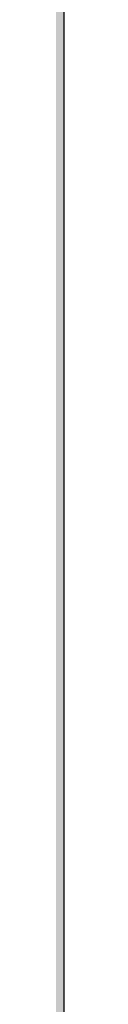
# Model space of a CAD drawing. Units: inches. Extents: x 2091 to 2899, y 967 to 2217.
# Tile 72 of 256: x 2212.144 to 2212.144, y 1102.499 to 1105.165. Entities that reach past the tile are written whole.
import ezdxf

# ---------------------------------------------------------------- set-up
doc = ezdxf.new("R2010")
doc.units = ezdxf.units.IN
doc.layers.add('A-ANNO-DIMS', color=2, linetype='Continuous', lineweight=18)
doc.layers.add('A-WALL-PATT', color=141, linetype='Continuous', lineweight=13, true_color=0xadddf7)
doc.styles.get("Standard").update_dxf_attribs({"font": 'arial.ttf'})
doc.dimstyles.new('ISO-25', dxfattribs={"dimtxt": 4, "dimasz": 4, "dimexe": 1.25, "dimexo": 0.625, "dimtad": 1, "dimdec": 0, "dimlunit": 3, "dimtxsty": 'Standard', "dimcen": 2.5, "dimadec": 0, "dimazin": 0, "dimtfac": 1, "dimtdec": 0, "dimtmove": 0, "dimatfit": 3, "dimfxl": 1, "dimarcsym": 0})

# ---------------------------------------------------------------- blocks, each defined once
blk = doc.blocks.new('*D71')
at = {"layer": 'A-ANNO-DIMS', "color": 0, "lineweight": -2, "transparency": 16777216}
for p, q in [((2212.1436, 1351.2941), (2212.1436, 969.4643)), ((2452.1436, 1351.2941), (2452.1436, 969.4643)), ((2216.1436, 970.7143), (2448.1436, 970.7143))]:
    blk.add_line(p, q, dxfattribs=at)
at = {"layer": 'A-ANNO-DIMS', "color": 0, "transparency": 16777216}
for points in [[(2216.1436, 971.381), (2216.1436, 970.0476), (2212.1436, 970.7143)], [(2448.1436, 971.381), (2448.1436, 970.0476), (2452.1436, 970.7143)]]:
    blk.add_solid(points, dxfattribs=at)
at = {"layer": 'Defpoints', "color": 0, "transparency": 16777216}
for p in [(2212.1436, 1351.9191), (2452.1436, 1351.9191), (2452.1436, 970.7143)]:
    blk.add_point(p, dxfattribs=at)
at = {"layer": 'A-ANNO-DIMS', "color": 0, "transparency": 16777216, "insert": (2332.1436, 973.3816), "char_height": 4, "attachment_point": 5}
blk.add_mtext('20\'-0"', dxfattribs=at)
blk = doc.blocks.new('*D75')
at = {"layer": 'A-ANNO-DIMS', "color": 0, "lineweight": -2, "transparency": 16777216}
for p, q in [((2212.1436, 1274.7941), (2212.1436, 969.4643)), ((2308.1436, 1274.7941), (2308.1436, 969.4643)), ((2216.1436, 970.7143), (2304.1436, 970.7143))]:
    blk.add_line(p, q, dxfattribs=at)
at = {"layer": 'A-ANNO-DIMS', "color": 0, "transparency": 16777216}
for points in [[(2216.1436, 971.381), (2216.1436, 970.0476), (2212.1436, 970.7143)], [(2304.1436, 971.381), (2304.1436, 970.0476), (2308.1436, 970.7143)]]:
    blk.add_solid(points, dxfattribs=at)
at = {"layer": 'Defpoints', "color": 0, "transparency": 16777216}
for p in [(2212.1436, 1275.4191), (2308.1436, 1275.4191), (2308.1436, 970.7143)]:
    blk.add_point(p, dxfattribs=at)
at = {"layer": 'A-ANNO-DIMS', "color": 0, "transparency": 16777216, "insert": (2260.1436, 973.3816), "char_height": 4, "attachment_point": 5}
blk.add_mtext('8\'-0"', dxfattribs=at)
blk = doc.blocks.new('*D91')
at = {"layer": 'A-ANNO-DIMS', "color": 0, "lineweight": -2, "transparency": 16777216}
for p, q in [((2211.6506, 1152.2471), (2098.3113, 1152.2471)), ((2099.5613, 1103.9191), (2099.5613, 1148.2471)), ((2211.5186, 1099.9191), (2098.3113, 1099.9191))]:
    blk.add_line(p, q, dxfattribs=at)
at = {"layer": 'A-ANNO-DIMS', "color": 0, "transparency": 16777216}
for points in [[(2098.8947, 1148.2471), (2100.228, 1148.2471), (2099.5613, 1152.2471)], [(2098.8947, 1103.9191), (2100.228, 1103.9191), (2099.5613, 1099.9191)]]:
    blk.add_solid(points, dxfattribs=at)
at = {"layer": 'Defpoints', "color": 0, "transparency": 16777216}
for p in [(2099.5613, 1152.2471), (2212.2756, 1152.2471), (2212.1436, 1099.9191)]:
    blk.add_point(p, dxfattribs=at)
at = {"layer": 'A-ANNO-DIMS', "color": 0, "transparency": 16777216, "insert": (2096.8681, 1126.0831), "char_height": 4, "attachment_point": 5, "rotation": 90}
blk.add_mtext('4\'-4 1/2"', dxfattribs=at)

msp = doc.modelspace()

# ---------------------------------------------------------------- hatches: boundary and pattern name
at = {"layer": 'A-WALL-PATT'}
h = msp.add_hatch(color=256, dxfattribs=at)
h.dxf.hatch_style = 1
h.paths.add_polyline_path([(2803.1436, 2050.9191), (2203.1436, 2050.9191), (2203.1436, 1090.9191), (2803.1436, 1090.9191)])
h.paths.add_polyline_path([(2635.7989, 1147.5405), (2674.5241, 1147.5405, 0.376086), (2678.5297, 1152.8802), (2678.5297, 1159.5565, 0.333335), (2674.5243, 1163.5618), (2674.5243, 1163.5619), (2674.5243, 1192.9344), (2635.806, 1192.9344), (2597.0876, 1192.9344), (2597.0876, 1163.5618, 0.333335), (2593.0823, 1159.5565), (2593.0823, 1152.8802, 0.376086), (2597.0879, 1147.5405)], flags=0)
h.paths.add_polyline_path([(2436.0104, 1278.2408, 0.000483), (2435.9526, 1278.215, -0.001328), (2435.9356, 1278.1117, -0.001711), (2436.1164, 1278.0408, 0.002185)], flags=0)
h.paths.add_polyline_path([(2794.1436, 1143.4191), (2794.1436, 1347.4191), (2543.3702, 1347.4191), (2543.3702, 1351.9191), (2794.1436, 1351.9191), (2794.1436, 1392.7136), (2793.9474, 1392.7136), (2793.9474, 1473.5369), (2794.1436, 1473.5369), (2794.1436, 1531.9191), (2650.1436, 1531.9191), (2650.1436, 1536.4191), (2794.1436, 1536.4191), (2794.1436, 1692.4191), (2609.3756, 1692.4191), (2609.3756, 1644.4191), (2604.8756, 1644.4191), (2604.8756, 1744.9191), (2609.3756, 1744.9191), (2609.3756, 1696.9191), (2794.1436, 1696.9191), (2794.1436, 1780.9191), (2609.6436, 1780.9191), (2493.8756, 1780.9191), (2493.8756, 1785.4191), (2609.6436, 1785.4191), (2794.1436, 1785.4191), (2794.1436, 1847.9388), (2793.9512, 1847.9388), (2793.9512, 1928.7622), (2794.1436, 1928.7622), (2794.1436, 1941.4191), (2614.1436, 1941.4191), (2614.1436, 1821.4191), (2609.6436, 1821.4191), (2609.6436, 1941.4191), (2392.1436, 1941.4191), (2392.1436, 1819.9191), (2387.6436, 1819.9191), (2387.6436, 1941.4191), (2212.1436, 1941.4191), (2212.1436, 1783.9191), (2392.1436, 1783.9191), (2392.1436, 1780.9191), (2212.1436, 1780.9191), (2212.1436, 1629.4191), (2387.6436, 1629.4191), (2387.6436, 1744.9191), (2392.1436, 1744.9191), (2392.1436, 1627.9191), (2317.1436, 1627.9191), (2317.1436, 1551.4191), (2317.1436, 1536.4191), (2459.3836, 1536.4191), (2459.3836, 1602.3965), (2463.8836, 1602.3965), (2463.8836, 1531.9191), (2456.6436, 1531.9191), (2456.6436, 1529.9191), (2452.1436, 1529.9191), (2452.1436, 1531.9191), (2312.6436, 1531.9191), (2312.6436, 1551.4191), (2306.1436, 1551.4191), (2306.1436, 1555.9191), (2308.1436, 1555.9191), (2308.1436, 1551.4191), (2312.6436, 1551.4191), (2312.6436, 1627.9191), (2212.1436, 1627.9191), (2212.1436, 1555.9191), (2270.1436, 1555.9191), (2270.1436, 1551.4191), (2212.1436, 1551.4191), (2212.1436, 1351.9191), (2272.1436, 1351.9191), (2272.1436, 1347.4191), (2212.1436, 1347.4191), (2212.1436, 1275.4191), (2308.1436, 1275.4191), (2308.1436, 1351.9191), (2452.1436, 1351.9191), (2452.1436, 1493.9191), (2456.6436, 1493.9191), (2456.6436, 1347.4191), (2312.6436, 1347.4191), (2312.6436, 1270.9191), (2212.1436, 1270.9191), (2212.1436, 1099.9191), (2281.2375, 1099.9191), (2282.871, 1110.9138), (2282.0083, 1116.9966), (2278.5577, 1121.4204), (2268.2056, 1128.0562), (2272.0876, 1128.0562), (2273.8129, 1131.927), (2279.4203, 1134.6919), (2285.0278, 1135.2449), (2287.6158, 1137.4568), (2288.0471, 1138.0098), (2289.3411, 1140.7747), (2291.0665, 1139.6687), (2292.3605, 1135.2449), (2295.3798, 1136.9038), (2296.2425, 1135.7979), (2297.1052, 1133.033), (2300.1246, 1138.0098), (2303.1439, 1138.0098), (2304.4379, 1135.7979), (2303.1439, 1133.586), (2306.5946, 1134.6919), (2307.8887, 1133.033), (2310.908, 1135.2449), (2313.9274, 1134.1389), (2315.6269, 1132.4271), (2308.32, 1117.5496), (2290.2038, 1109.8079), (2288.9098, 1103.1721), (2289.2723, 1099.9191), (2434.9182, 1099.9191), (2431.5932, 1124.7881), (2429.9302, 1169.5531), (2430.9272, 1240.5197), (2435.6589, 1238.1861), (2437.1352, 1196.5541), (2438.7982, 1143.9731), (2442.6782, 1111.9981), (2446.5582, 1099.9191), (2794.1436, 1099.9191), (2794.1436, 1138.9191), (2548.0324, 1138.9191), (2548.0324, 1143.4191), (2548.0324, 1148.8191), (2546.6685, 1148.0316), (2528.6857, 1179.1786, 0.256256), (2512.0324, 1148.8191), (2512.0324, 1143.4191), (2512.0324, 1138.9191), (2507.5324, 1138.9191), (2507.5324, 1143.4191), (2507.5324, 1148.8191, 0.256256), (2490.8792, 1179.1786), (2472.8964, 1148.0316), (2471.5324, 1148.8191), (2471.5324, 1143.4191), (2467.0324, 1143.4191), (2467.0324, 1269.9458, 0.039061), (2460.91, 1273.5801), (2467.0324, 1273.5801), (2467.0324, 1286.3254, 0.014511), (2465.2162, 1286.7619), (2467.0324, 1287.0526), (2467.0324, 1323.4191), (2471.5324, 1323.4191), (2471.5324, 1148.8191), (2489.5324, 1179.996), (2490.8964, 1179.2085), (2490.8792, 1179.1786, -0.256256), (2507.5324, 1148.8191), (2507.5324, 1143.4191), (2512.0324, 1143.4191), (2512.0324, 1148.8191, -0.256256), (2528.6857, 1179.1786), (2528.6685, 1179.2085), (2530.0324, 1179.996), (2548.0324, 1148.8191), (2548.0324, 1143.4191)], flags=16)
h.paths.add_polyline_path([(2607.7685, 1200.9451), (2607.7685, 1265.0306), (2597.0876, 1281.052), (2619.7846, 1281.052), (2627.7953, 1337.1269), (2635.7989, 1337.1269), (2643.8167, 1337.1269), (2651.8274, 1281.052), (2674.5243, 1281.052), (2663.8434, 1265.0306), (2663.8434, 1200.9451), (2635.806, 1200.9451)], flags=0)
edge = h.paths.add_edge_path(flags=0)
edge.add_ellipse((13303.8962, 1272.9987), major_axis=(-10595.313, 0), ratio=0.8423038701, start_angle=0.62823722, end_angle=0.6465541, ccw=False)
edge.add_ellipse((2711.7004, 1156.8527), major_axis=(2.2198, 0), ratio=0.842304, start_angle=111.5352, end_angle=180.6282, ccw=False)
edge.add_ellipse((13303.1563, 1272.9987), major_axis=(-10593.0263, 0), ratio=0.8423038695, start_angle=0.52827147, end_angle=0.6465541, ccw=False)
edge.add_line((2710.7646, 1175.3333), (2710.13, 1175.3333))
edge.add_ellipse((2710.13, 1176.5798), major_axis=(1.4798, 0), ratio=0.842304, start_angle=180, end_angle=270, ccw=False)
edge.add_line((2708.6501, 1176.5798), (2708.6501, 1200.7829))
edge.add_ellipse((2710.13, 1200.7829), major_axis=(1.4798, 0), ratio=0.842304, start_angle=90, end_angle=180, ccw=False)
edge.add_line((2710.13, 1202.0294), (2710.4651, 1202.0294))
edge.add_ellipse((13303.1563, 1272.9987), major_axis=(-10593.0263, 0), ratio=0.8423038695, start_angle=-0.09022909, end_angle=0.38386678, ccw=False)
edge.add_ellipse((2710.13, 1290.927), major_axis=(-1.4798, 0), ratio=0.842304, start_angle=0, end_angle=90, ccw=False)
edge.add_line((2708.6501, 1290.927), (2708.6501, 1315.1302))
edge.add_ellipse((2710.13, 1315.1302), major_axis=(-1.4798, 0), ratio=0.842304, start_angle=-90, end_angle=0, ccw=False)
edge.add_line((2710.13, 1316.3767), (2710.7063, 1316.3767))
edge.add_ellipse((3238.4017, 1296.2896), major_axis=(528.234, 0), ratio=0.84230387, start_angle=176.349572, end_angle=177.82005, ccw=False)
edge.add_ellipse((2775.063, 1071.4507), major_axis=(313.3078, 0), ratio=0.84230387, start_angle=102.125966, end_angle=103.780529, ccw=False)
edge.add_ellipse((2775.063, 1078.3057), major_axis=(-305.3029, 0), ratio=0.84230387, start_angle=-79.790461, end_angle=-77.555373, ccw=False)
edge.add_ellipse((2695.1418, 1541.9754), major_axis=(-250.9602, 0), ratio=0.84230387, start_angle=99.256566, end_angle=102.554933)
edge.add_line((2741.4103, 1334.2143), (2747.1325, 1337.3785))
edge.add_ellipse((2747.5386, 1336.8575), major_axis=(-0.7399, 0), ratio=0.842304, start_angle=270, end_angle=307.9331, ccw=False)
edge.add_ellipse((2747.5386, 1336.8575), major_axis=(-0.7399, 0), ratio=0.842304, start_angle=232.0669, end_angle=270, ccw=False)
edge.add_line((2747.9447, 1337.3785), (2753.6669, 1334.2143))
edge.add_ellipse((2799.9355, 1541.9754), major_axis=(250.9602, 0), ratio=0.84230387, start_angle=257.445067, end_angle=260.743434)
edge.add_ellipse((2720.0142, 1078.3057), major_axis=(305.3029, 0), ratio=0.84230387, start_angle=77.555373, end_angle=79.790461, ccw=False)
edge.add_ellipse((2720.0142, 1071.4507), major_axis=(-313.3078, 0), ratio=0.84230387, start_angle=256.219471, end_angle=257.874034, ccw=False)
edge.add_ellipse((2256.6755, 1296.2896), major_axis=(-528.234, 0), ratio=0.84230387, start_angle=182.17995, end_angle=183.650428, ccw=False)
edge.add_line((2784.3709, 1316.3767), (2784.9472, 1316.3767))
edge.add_ellipse((2784.9472, 1315.1302), major_axis=(1.4798, 0), ratio=0.842304, start_angle=0, end_angle=90, ccw=False)
edge.add_line((2786.4271, 1315.1302), (2786.4271, 1290.927))
edge.add_ellipse((2784.9472, 1290.927), major_axis=(1.4798, 0), ratio=0.842304, start_angle=270, end_angle=360, ccw=False)
edge.add_ellipse((-7808.0791, 1272.9987), major_axis=(10593.0263, 0), ratio=0.8423038695, start_angle=-0.38386678, end_angle=0.09022909, ccw=False)
edge.add_line((2784.6122, 1202.0294), (2784.9472, 1202.0294))
edge.add_ellipse((2784.9472, 1200.7829), major_axis=(1.4798, 0), ratio=0.842304, start_angle=0, end_angle=90, ccw=False)
edge.add_line((2786.4271, 1200.7829), (2786.4271, 1176.5798))
edge.add_ellipse((2784.9472, 1176.5798), major_axis=(-1.4798, 0), ratio=0.842304, start_angle=90, end_angle=180, ccw=False)
edge.add_line((2784.9472, 1175.3333), (2784.3126, 1175.3333))
edge.add_ellipse((-7808.0791, 1272.9987), major_axis=(10593.0263, 0), ratio=0.8423038695, start_angle=-0.6186432, end_angle=-0.52827147, ccw=False)
edge.add_ellipse((2783.3768, 1156.8527), major_axis=(-2.2198, 0), ratio=0.842304, start_angle=179.3718, end_angle=248.4648, ccw=False)
edge.add_ellipse((-7808.819, 1272.9987), major_axis=(-10595.313, 0), ratio=0.8423038658, start_angle=179.35344592, end_angle=179.3717628, ccw=False)
edge.add_ellipse((2780.2973, 1153.5008), major_axis=(-5.2464, 0), ratio=0.842304, start_angle=90, end_angle=179.3534, ccw=False)
edge.add_line((2780.2973, 1149.0817), (2714.7799, 1149.0817))
edge.add_ellipse((2714.7799, 1153.5008), major_axis=(5.2464, 0), ratio=0.842304, start_angle=180.6466, end_angle=270, ccw=False)
edge = h.paths.add_edge_path(flags=0)
edge.add_line((2718.1874, 1151.0078), (2718.1874, 1170.4724))
edge.add_ellipse((2721.1471, 1170.4724), major_axis=(-2.9597, 0), ratio=0.842304, start_angle=-90, end_angle=0, ccw=False)
edge.add_line((2721.1471, 1172.9653), (2773.9302, 1172.9653))
edge.add_ellipse((2773.9302, 1170.4724), major_axis=(-2.9597, 0), ratio=0.842304, start_angle=180, end_angle=270, ccw=False)
edge.add_line((2776.8899, 1170.4724), (2776.8899, 1151.0078))
edge.add_line((2776.8899, 1151.0078), (2718.1874, 1151.0078))
edge = h.paths.add_edge_path(flags=0)
edge.add_line((2718.1874, 1180.2342), (2718.1874, 1199.0578))
edge.add_ellipse((2747.5386, 1320.3986), major_axis=(147.0179, 0), ratio=0.84230387, start_angle=256.401865, end_angle=283.598135)
edge.add_line((2776.8899, 1199.0578), (2776.8899, 1180.2342))
edge.add_ellipse((2747.5386, 1301.575), major_axis=(147.0179, 0), ratio=0.84230387, start_angle=256.401865, end_angle=283.598135, ccw=False)
edge = h.paths.add_edge_path(flags=0)
edge.add_ellipse((13303.1563, 1272.9987), major_axis=(-10591.5465, 0), ratio=0.8423038696, start_angle=0.05559431, end_angle=0.37776419, ccw=False)
edge.add_line((2711.6169, 1262.7217), (2715.6674, 1249.4954))
edge.add_ellipse((6413.892, 1241.6919), major_axis=(-3698.2362, 0), ratio=0.84230387, start_angle=-0.1208974, end_angle=0.3640763)
edge.add_line((2715.761, 1218.1925), (2711.9343, 1203.1674))
edge = h.paths.add_edge_path(flags=0)
edge.add_line((2718.1874, 1251.0746), (2716.0025, 1267.4504))
edge.add_ellipse((2742.1512, 1202.1895), major_axis=(81.7726, 0), ratio=0.8423039, start_angle=94.277421, end_angle=111.834954, ccw=False)
edge.add_line((2737.0097, 1270.9306), (2758.0675, 1270.9306))
edge.add_ellipse((2752.9261, 1202.1895), major_axis=(81.7726, 0), ratio=0.8423039, start_angle=68.165046, end_angle=85.722579, ccw=False)
edge.add_line((2779.0747, 1267.4504), (2776.8899, 1251.0746))
edge.add_ellipse((2750.3381, 1187.8854), major_axis=(79.5797, 0), ratio=0.8423039, start_angle=67.208085, end_angle=85.12993)
edge.add_line((2756.0347, 1254.7437), (2739.0426, 1254.7437))
edge.add_ellipse((2744.7392, 1187.8854), major_axis=(79.5797, 0), ratio=0.8423039, start_angle=94.87007, end_angle=112.791915)
edge = h.paths.add_edge_path(flags=0)
edge.add_line((2783.1429, 1203.1674), (2779.3162, 1218.1925))
edge.add_ellipse((-918.8147, 1241.6919), major_axis=(3698.2362, 0), ratio=0.84230387, start_angle=-0.3640763, end_angle=0.1208974)
edge.add_line((2779.4098, 1249.4954), (2783.4604, 1262.7217))
edge.add_ellipse((-7808.0791, 1272.9987), major_axis=(-10591.5465, 0), ratio=0.8423038695, start_angle=179.62223581, end_angle=179.94440569, ccw=False)
edge = h.paths.add_edge_path(flags=0)
edge.add_ellipse((2734.2009, 1286.6904), major_axis=(-0.3566, 6.3401), ratio=0.603834, start_angle=89.00201, end_angle=253.65741, ccw=False)
edge.add_line((2730.369, 1286.5418), (2730.369, 1301.352))
edge.add_line((2730.369, 1301.352), (2735.9133, 1305.2148))
edge.add_ellipse((2736.3849, 1304.7346), major_axis=(0.7399, 0), ratio=0.842304, start_angle=90, end_angle=134.4802, ccw=False)
edge.add_line((2736.3849, 1305.3578), (2738.0328, 1305.3578))
edge.add_line((2738.0328, 1305.3578), (2738.0328, 1307.7079))
edge.add_ellipse((2794.2016, 1307.7079), major_axis=(56.1689, 0), ratio=0.8423039, start_angle=150.56143, end_angle=180, ccw=False)
edge.add_ellipse((2700.8756, 1307.7079), major_axis=(-56.1689, 0), ratio=0.8423039, start_angle=180, end_angle=209.43857, ccw=False)
edge.add_line((2757.0444, 1307.7079), (2757.0444, 1305.3578))
edge.add_line((2757.0444, 1305.3578), (2758.6923, 1305.3578))
edge.add_ellipse((2758.6923, 1304.7346), major_axis=(-0.7399, 0), ratio=0.842304, start_angle=225.5198, end_angle=270, ccw=False)
edge.add_line((2759.1639, 1305.2148), (2764.7082, 1301.352))
edge.add_line((2764.7082, 1301.352), (2764.7082, 1286.5418))
edge.add_ellipse((2760.8763, 1286.6904), major_axis=(0.3566, 6.3401), ratio=0.603834, start_angle=106.34259, end_angle=270.99799, ccw=False)
edge.add_line((2757.0444, 1285.7971), (2757.0444, 1307.7079))
edge.add_ellipse((2700.8756, 1307.7079), major_axis=(-56.1689, 0), ratio=0.8423039, start_angle=180, end_angle=209.43857)
edge.add_ellipse((2794.2016, 1307.7079), major_axis=(56.1689, 0), ratio=0.8423039, start_angle=150.56143, end_angle=180)
edge.add_line((2738.0328, 1307.7079), (2738.0328, 1285.7971))
h.paths.add_polyline_path([(2417.8123, 1104.4497), (2413.4923, 1102.5297), (2410.6123, 1103.9697), (2409.1723, 1106.3697), (2407.2523, 1107.3297), (2406.2923, 1109.7297), (2405.3323, 1114.0497), (2405.3323, 1117.8897), (2406.2923, 1120.1297), (2407.2523, 1119.8097), (2408.8483, 1118.3277), (2410.1739, 1119.4242), (2410.2113, 1120.4057), (2411.0407, 1121.4191), (2410.6993, 1119.8587), (2410.1739, 1119.4242), (2410.0885, 1117.1761), (2411.1328, 1116.2063), (2413.9723, 1119.3297), (2416.8523, 1120.7697), (2416.8697, 1120.7988), (2417.0351, 1119.4051), (2417.8962, 1118.1434), (2418.2923, 1118.3697), (2419.5444, 1120.0393), (2419.3609, 1118.3875), (2419.0321, 1119.3562), (2418.3989, 1118.5119), (2419.2523, 1114.5297), (2418.7941, 1107.1988)], flags=0)
h.paths.add_polyline_path([(2508.8702, 1347.4191), (2508.3702, 1347.4191), (2508.3702, 1351.9191), (2508.8702, 1351.9191)], flags=0)
h.paths.add_polyline_path([(2473.3702, 1347.4191), (2472.3702, 1347.4191), (2467.8702, 1347.4191), (2467.8702, 1455.4191), (2472.3702, 1455.4191), (2472.3702, 1352.4191), (2473.3702, 1352.4191)], flags=0)
h.paths.add_polyline_path([(2352.1062, 1217.4462), (2349.2262, 1218.8862), (2347.7862, 1221.2862), (2345.8662, 1222.2462), (2344.9062, 1224.6462), (2343.9462, 1228.9662), (2343.9462, 1232.8062), (2344.9062, 1235.0462), (2345.8662, 1234.7262), (2347.4623, 1233.2442), (2348.7879, 1234.3407), (2348.8252, 1235.3222), (2349.6547, 1236.3355), (2349.3132, 1234.7752), (2348.7879, 1234.3407), (2348.7024, 1232.0926), (2349.7468, 1231.1228), (2352.5862, 1234.2462), (2355.4662, 1235.6862), (2355.4837, 1235.7153), (2355.649, 1234.3216), (2356.5102, 1233.0599), (2356.9062, 1233.2862), (2358.1584, 1234.9558), (2357.9749, 1233.304), (2357.6461, 1234.2726), (2357.0129, 1233.4284), (2357.8662, 1229.4462), (2357.4081, 1222.1153), (2356.4262, 1219.3662)], flags=0)
h.paths.add_polyline_path([(2348.2968, 1112.2244), (2347.0138, 1112.3104), (2345.5298, 1114.1274), (2345.7318, 1115.8584), (2346.8118, 1116.9824), (2346.8118, 1114.6464), (2345.8668, 1114.2144), (2346.8798, 1114.3004)], flags=0)
h.paths.add_polyline_path([(2347.0138, 1110.9264), (2346.2718, 1110.4934), (2346.6098, 1111.1864)], flags=0)
h.paths.add_polyline_path([(2345.8668, 1118.1944), (2345.5298, 1117.3294), (2343.7078, 1118.0214), (2344.3828, 1118.6264)], flags=0)
h.paths.add_polyline_path([(2346.6768, 1109.2824), (2346.0698, 1108.0714), (2345.8668, 1110.0614)], flags=0)
h.paths.add_polyline_path([(2345.0568, 1119.7514), (2343.6398, 1119.7514), (2343.9778, 1121.1354)], flags=0)
h.paths.add_polyline_path([(2345.2598, 1116.5504), (2345.1248, 1115.8584), (2344.9218, 1115.6854), (2344.7198, 1116.3774)], flags=0)
h.paths.add_polyline_path([(2345.6648, 1112.3104), (2345.4618, 1111.5324), (2344.0448, 1111.9644), (2344.6518, 1112.5704)], flags=0)
h.paths.add_polyline_path([(2345.1918, 1113.3494), (2344.4498, 1113.8684), (2344.7198, 1114.3874)], flags=0)
h.paths.add_polyline_path([(2344.6518, 1116.8094), (2344.1798, 1115.6854), (2344.6518, 1115.3394), (2343.9098, 1114.9064), (2343.0328, 1115.9444), (2343.6398, 1116.4634)], flags=0)
h.paths.add_polyline_path([(2345.8668, 1106.6864), (2344.9898, 1105.5624), (2344.5168, 1106.6004)], flags=0)
h.paths.add_polyline_path([(2344.8548, 1110.0614), (2344.5168, 1109.2824), (2344.1128, 1109.7154)], flags=0)
h.paths.add_polyline_path([(2344.0448, 1113.5224), (2343.4378, 1113.0894), (2342.7628, 1113.9544)], flags=0)
h.paths.add_polyline_path([(2344.3148, 1111.0124), (2342.9648, 1110.3204), (2342.9648, 1111.0994)], flags=0)
h.paths.add_polyline_path([(2345.1248, 1104.6974), (2344.5848, 1103.7454), (2344.4498, 1104.2644)], flags=0)
h.paths.add_polyline_path([(2342.8298, 1121.2224), (2341.7498, 1120.5304), (2340.5358, 1121.0494), (2340.1308, 1121.8284), (2340.6708, 1122.9524), (2341.1428, 1121.8284), (2341.6148, 1122.0014)], flags=0)
h.paths.add_polyline_path([(2342.9648, 1119.7514), (2343.0328, 1118.4534), (2342.0878, 1118.0214), (2342.0198, 1119.4914)], flags=0)
h.paths.add_polyline_path([(2342.6948, 1116.8964), (2341.9528, 1116.6364), (2342.0198, 1117.3294)], flags=0)
h.paths.add_polyline_path([(2343.0328, 1112.2244), (2342.0198, 1111.7914), (2341.5478, 1112.2244), (2342.3578, 1113.3494)], flags=0)
h.paths.add_polyline_path([(2343.7748, 1104.4374), (2342.6278, 1102.8804), (2342.6948, 1104.6104), (2343.4378, 1105.1294)], flags=0)
h.paths.add_polyline_path([(2342.0198, 1115.0794), (2340.8058, 1115.5124), (2340.9408, 1116.3774)], flags=0)
h.paths.add_polyline_path([(2341.4808, 1120.0974), (2341.4808, 1119.4054), (2341.0758, 1119.5784), (2341.1428, 1120.0974)], flags=0)
h.paths.add_polyline_path([(2341.8178, 1114.4734), (2340.9408, 1113.0894), (2340.8058, 1114.5604)], flags=0)
h.paths.add_polyline_path([(2341.1428, 1118.5404), (2340.9408, 1116.9824), (2339.0508, 1117.6754), (2339.0508, 1118.6264)], flags=0)
h.paths.add_polyline_path([(2342.6948, 1101.6684), (2341.9528, 1101.8414), (2342.5598, 1102.3614)], flags=0)
h.paths.add_polyline_path([(2340.3328, 1119.6654), (2338.4438, 1119.5784), (2337.9038, 1120.3574), (2339.6578, 1120.6164)], flags=0)
h.paths.add_polyline_path([(2340.3328, 1115.3394), (2340.0628, 1113.6954), (2339.3878, 1115.3394)], flags=0)
h.paths.add_polyline_path([(2341.8178, 1103.8314), (2341.5478, 1102.8804), (2341.1428, 1103.6584)], flags=0)
h.paths.add_polyline_path([(2339.0508, 1122.8664), (2337.2958, 1121.8284), (2337.0938, 1123.1254), (2337.7688, 1123.8184)], flags=0)
h.paths.add_polyline_path([(2339.1178, 1121.7414), (2338.8478, 1121.2224), (2338.1738, 1121.0494), (2338.3758, 1121.5684)], flags=0)
h.paths.add_polyline_path([(2339.1858, 1119.3194), (2338.6458, 1118.7134), (2338.2408, 1118.1074), (2338.2408, 1118.8864)], flags=0)
h.paths.add_polyline_path([(2341.1428, 1101.9284), (2340.6028, 1101.2364), (2340.0628, 1101.8414), (2340.6028, 1102.3614)], flags=0)
h.paths.add_polyline_path([(2337.6338, 1117.7614), (2336.6208, 1118.2804), (2337.2958, 1118.9724)], flags=0)
h.paths.add_polyline_path([(2336.8238, 1119.5784), (2334.7988, 1118.9724), (2335.2038, 1120.3574), (2336.5538, 1120.8764)], flags=0)
h.paths.add_polyline_path([(2339.1178, 1100.4574), (2337.3638, 1100.5434), (2336.7558, 1101.2364)], flags=0)
h.paths.add_polyline_path([(2336.3508, 1122.4334), (2336.0138, 1121.9144), (2334.9338, 1122.4334), (2334.5288, 1123.4714), (2335.7438, 1122.7794)], flags=0)
h.paths.add_polyline_path([(2334.7318, 1120.8764), (2334.2588, 1120.3574), (2334.0568, 1120.7894), (2334.5968, 1121.3084)], flags=0)
h.paths.add_polyline_path([(2334.4618, 1122.1744), (2332.5718, 1121.3084), (2331.3568, 1122.1744), (2332.0998, 1122.8664)], flags=0)
h.paths.add_polyline_path([(2334.2588, 1118.5404), (2333.3818, 1118.4534), (2333.6518, 1119.3194)], flags=0)
h.paths.add_polyline_path([(2335.5418, 1102.2744), (2334.1918, 1102.6204), (2335.2718, 1103.3124)], flags=0)
h.paths.add_polyline_path([(2332.7068, 1119.6654), (2331.6948, 1120.4434), (2332.5048, 1120.7894)], flags=0)
h.paths.add_polyline_path([(2334.7318, 1101.1494), (2333.5168, 1101.5824), (2333.9888, 1101.7554)], flags=0)
h.paths.add_polyline_path([(2332.6398, 1116.6364), (2331.0868, 1116.2904), (2331.9648, 1118.1944)], flags=0)
h.paths.add_polyline_path([(2330.7498, 1121.5684), (2330.2768, 1120.2704), (2328.5228, 1119.3194), (2328.9948, 1121.0494)], flags=0)
h.paths.add_polyline_path([(2330.7498, 1118.6264), (2330.0078, 1117.5024), (2329.8728, 1118.0214)], flags=0)
h.paths.add_polyline_path([(2332.0998, 1102.3614), (2330.5468, 1102.0144), (2331.6948, 1102.9664)], flags=0)
h.paths.add_polyline_path([(2329.5348, 1113.6084), (2329.0628, 1112.3104), (2328.5898, 1113.3494)], flags=0)
h.paths.add_polyline_path([(2328.3878, 1117.8484), (2327.5098, 1116.5504), (2327.1728, 1117.7614)], flags=0)
h.paths.add_polyline_path([(2329.7378, 1106.5134), (2329.5348, 1105.3024), (2328.2528, 1106.0814)], flags=0)
h.paths.add_polyline_path([(2328.6578, 1114.3874), (2328.0498, 1114.1274), (2328.3198, 1114.9064)], flags=0)
h.paths.add_polyline_path([(2328.3198, 1112.2244), (2327.1058, 1112.1374), (2326.7008, 1112.6564)], flags=0)
h.paths.add_polyline_path([(2326.9028, 1115.2524), (2326.7008, 1114.1274), (2325.2158, 1113.6084), (2326.0928, 1115.3394)], flags=0)
h.paths.add_polyline_path([(2326.6328, 1108.3304), (2326.0928, 1107.3794), (2325.8908, 1108.5034), (2326.4978, 1109.1094)], flags=0)
h.paths.add_polyline_path([(2615.1436, 1531.9191), (2609.6436, 1531.9191), (2609.6436, 1620.4191), (2614.1436, 1620.4191), (2614.1436, 1536.4191), (2615.1436, 1536.4191)], flags=0)
h.paths.add_polyline_path([(2545.1436, 1563.4191), (2464.1436, 1563.4191), (2464.1436, 1632.4191), (2509.1436, 1632.4191), (2509.1436, 1627.9191), (2509.1436, 1603.9191), (2468.6436, 1603.9191), (2468.6436, 1567.9191), (2540.6436, 1567.9191), (2540.6436, 1591.9191), (2545.1436, 1591.9191)], flags=0)
h.paths.add_polyline_path([(2388.969, 1549.9857), (2357.4342, 1549.9857), (2357.4342, 1623.3608), (2399.3628, 1623.3608), (2435.6895, 1623.3608), (2435.5925, 1602.5593), (2435.5925, 1602.3965), (2388.969, 1602.3965)], flags=0)
h.paths.add_polyline_path([(2388.8806, 1555.8092), (2374.9044, 1555.8092), (2374.9044, 1600.5716), (2374.9044, 1615.4576), (2406.3509, 1615.4576), (2406.3509, 1618.9394), (2412.1743, 1615.4576), (2406.3509, 1611.9759), (2406.3509, 1615.4576), (2388.8806, 1615.4576)], flags=0)
h.paths.add_polyline_path([(2568.8756, 1644.4191), (2453.3756, 1644.4191), (2453.3756, 1785.4191), (2457.8756, 1785.4191), (2457.8756, 1648.9191), (2568.8756, 1648.9191)], flags=0)
h.paths.add_polyline_path([(2212.1436, 1945.9191), (2212.1436, 2041.9191), (2794.1436, 2041.9191), (2794.1436, 1945.9191)], flags=16)
h.paths.add_polyline_path([(2271.0827, 1964.3172), (2776.853, 1964.3172), (2776.853, 2037.1696), (2271.0827, 2037.1696)], flags=8)
h.paths.add_polyline_path([(2380.6493, 1536.8241), (2461.0408, 1536.8241), (2461.0408, 1554.6526), (2380.6493, 1554.6526)], flags=8)
h.paths.add_polyline_path([(2240.7557, 1609.7255), (2309.1858, 1609.7255), (2309.1858, 1617.6982), (2240.7557, 1617.6982)], flags=8)
h.paths.add_polyline_path([(2212.6773, 1313.5041), (2282.5915, 1313.5041), (2282.5915, 1322.7452), (2212.6773, 1322.7452)], flags=8)
h.paths.add_polyline_path([(2457.112, 1114.7786), (2558.4816, 1114.7786), (2558.4816, 1142.2197), (2457.112, 1142.2197)], flags=8)
h.paths.add_polyline_path([(2473.4423, 1273.0101), (2604.6412, 1273.0101), (2604.6412, 1318.3469), (2473.4423, 1318.3469)], flags=8)
h.paths.add_polyline_path([(2638.8763, 1626.9774), (2684.2504, 1627.9767), (2684.0385, 1637.5975), (2638.6644, 1636.5982)], flags=8)
h.paths.add_polyline_path([(2537.5906, 1453.7934), (2628.3895, 1453.7934), (2628.3895, 1475.3448), (2537.5906, 1475.3448)], flags=8)
h.paths.add_polyline_path([(2504.1376, 1714.6324), (2554.6472, 1714.6324), (2554.6472, 1730.2377), (2504.1376, 1730.2377)], flags=8)
h.paths.add_polyline_path([(2487.5012, 1575.6519), (2535.0971, 1575.6519), (2535.0971, 1598.3776), (2487.5012, 1598.3776)], flags=8)
h.paths.add_polyline_path([(2709.0994, 1735.7103), (2740.0166, 1735.7103), (2740.0166, 1749.9376), (2709.0994, 1749.9376)], flags=8)
h.paths.add_polyline_path([(2442.4384, 1792.1717), (2564.7288, 1792.1717), (2564.7288, 1842.0002), (2442.4384, 1842.0002)], flags=8)
h.paths.add_polyline_path([(2655.8158, 1809.6441), (2789.5201, 1806.6938), (2790.085, 1832.2916), (2656.3806, 1835.2419)], flags=8)
h.paths.add_polyline_path([(2234.8427, 1797.7201), (2368.5929, 1794.7689), (2369.1607, 1820.5041), (2235.4106, 1823.4554)], flags=8)
h.paths.add_polyline_path([(2245.1385, 1644.0063), (2398.4277, 1640.6239), (2398.9948, 1666.3248), (2245.7056, 1669.7073)], flags=8)
h.paths.add_polyline_path([(2306.1428, 1431.1685), (2413.7683, 1428.7937), (2414.3331, 1454.3915), (2306.7077, 1456.7664)], flags=8)
h.paths.add_polyline_path([(2306.8346, 1458.2331), (2393.3805, 1456.3234), (2393.9328, 1481.3544), (2307.3869, 1483.2641)], flags=8)

# ---------------------------------------------------------------- dimensions: what is measured, and where the dimension line sits
at = {"layer": 'A-ANNO-DIMS'}
for base, p1, p2, picture, middle in [((2452.1436, 970.7143), (2212.1436, 1351.9191), (2452.1436, 1351.9191), '*D71', (2332.1436, 973.3816)), ((2308.1436, 970.7143), (2212.1436, 1275.4191), (2308.1436, 1275.4191), '*D75', (2260.1436, 973.3816))]:
    dim = msp.add_linear_dim(base=base, p1=p1, p2=p2, dimstyle='ISO-25', override={"dimdec": 1, "dimlfac": 1, "dimrnd": 0, "dimzin": 1, "dimdsep": 46, "dimlunit": 4, "dimfrac": 2}, dxfattribs=at)
    dim.commit()
    dim.dimension.update_dxf_attribs({"geometry": picture, "text_midpoint": middle})
dim = msp.add_linear_dim(base=(2099.5613, 1152.2471), p1=(2212.1436, 1099.9191), p2=(2212.2756, 1152.2471), angle=90, dimstyle='ISO-25', override={"dimdec": 1, "dimlfac": 1, "dimrnd": 0, "dimzin": 1, "dimdsep": 46, "dimlunit": 4, "dimfrac": 2}, dxfattribs=at)
dim.commit()
dim.dimension.update_dxf_attribs({"geometry": '*D91', "text_midpoint": (2096.8681, 1126.0831)})

doc.saveas('drawing.dxf')
